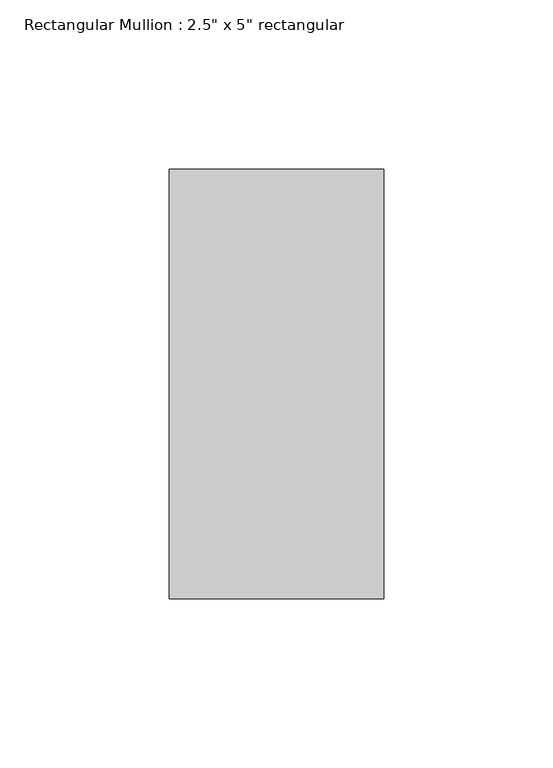
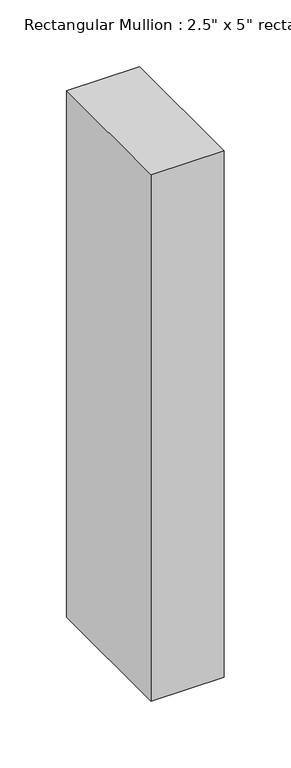
"""IFC4 building model written with IfcOpenShell, lengths in millimetres: member geometry."""

from ifc_helpers import new_model, si_unit, frame, origin, place, context, project, spatial, polyline, outline, extrude, source, transform, mapped, element, save


def member_86d06fe4(model_context):
    return source(origin(), model_context, "Body", "SweptSolid", [
        extrude(outline(polyline([(0.0, 63.5), (0.0, -63.5), (-63.5, -63.5), (-63.5, 63.5), (0.0, 63.5)])), frame((0.0, 0.0, -482.6), z_axis=(0.0, 0.0, 1.0), x_axis=(1.0, 0.0, 0.0)), (0.0, 0.0, 1.0), 482.6),
    ])


if __name__ == "__main__":
    model = new_model("IFC4")
    model_context = context("Model", 3, world=origin())
    ifc_project = project(units=[si_unit("LENGTHUNIT", "METRE", prefix="MILLI")], contexts=[model_context])
    site = spatial("IfcSite", under=ifc_project)
    building = spatial("IfcBuilding", under=site)
    placement = place(None, origin())
    member_shape = member_86d06fe4(model_context)
    element("IfcMember", 1, ObjectType="Rectangular Mullion : 2.5\" x 5\" rectangular", at=placement, inside=building, context=model_context, shape_type="MappedRepresentation", body=[
        mapped(member_shape, transform((0.0, 0.0, 0.0), x_axis=(1.0, 0.0, 0.0), y_axis=(0.0, 1.0, 0.0), z_axis=(0.0, 0.0, 1.0))),
    ])
    save(model, "model.ifc")

# Revit data of these elements
# Type "Rectangular Mullion : 2.5\" x 5\" rectangular"
#   built-in parameter 1007304 = 0.416667 (stored number, unit not read)
#   built-in parameter 1007301 = 0.104167 (stored number, unit not read)
#   built-in parameter 1007300 = 0.104167 (stored number, unit not read)
# Element 1 (IfcMember, "Rectangular Mullion : 2.5\" x 5\" rectangular")
#   Materials on its faces: "door colour"
# Materials
#   "door colour": class "Generic", colour RGB 120 120 120, transparency 0, Cost = 0
